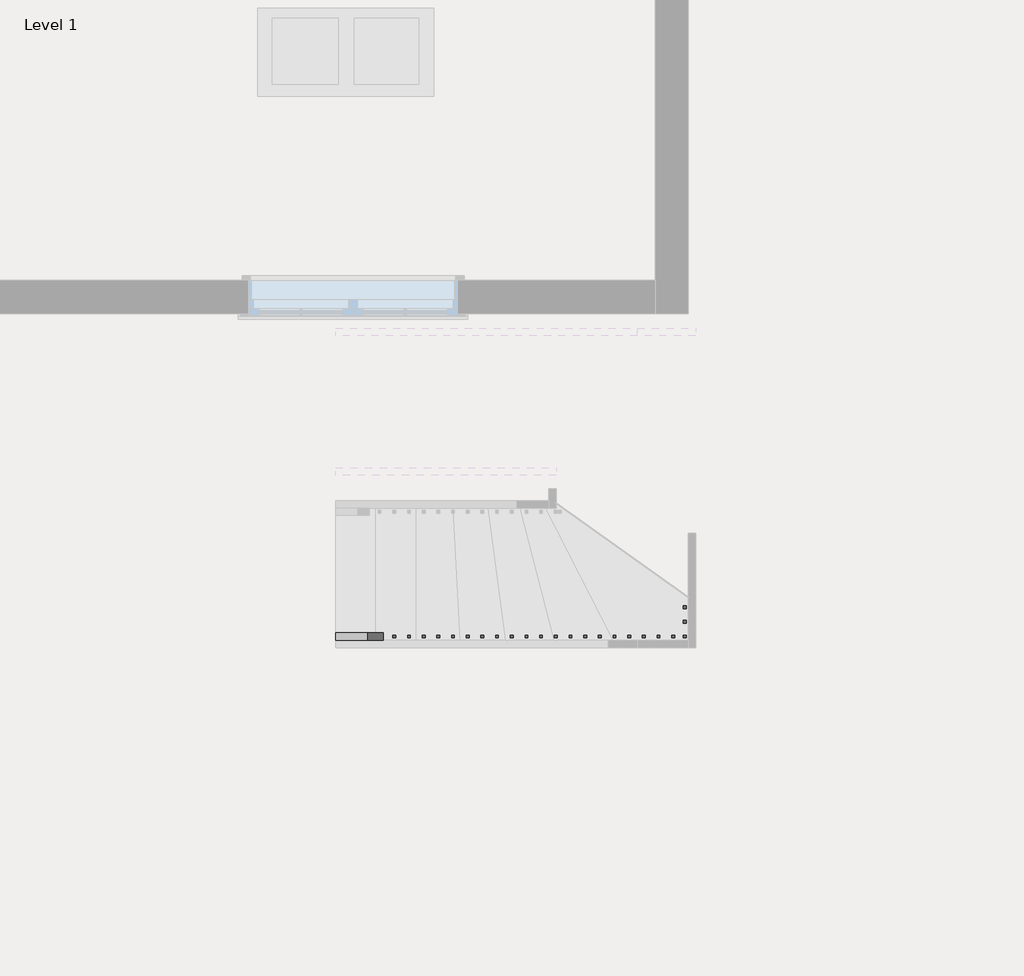
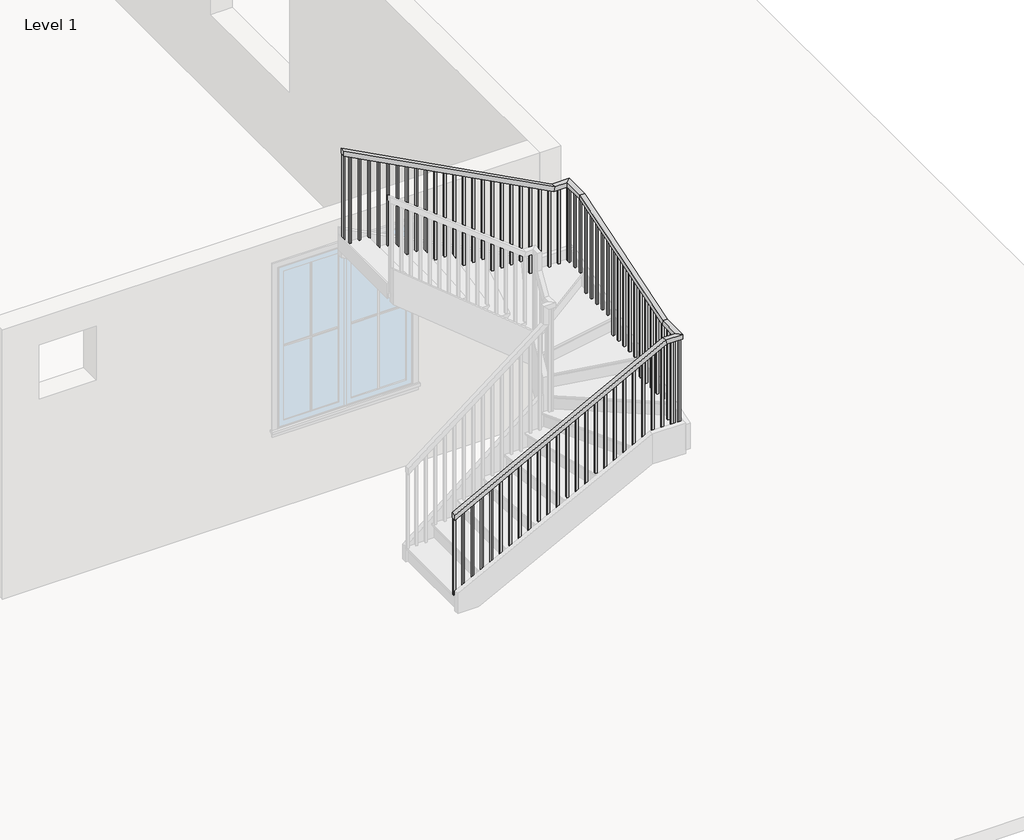
# One storey, part 2 of 3: 1 railing.
"""IFC4 building model written with IfcOpenShell, lengths in millimetres."""

from ifc_helpers import new_model, si_unit, frame, origin, place, context, project, spatial, polyline, outline, extrude, faceted_brep, element, save

model = new_model("IFC4")

# Units and contexts
model_context = context("Model", 3, world=origin())
ifc_project = project(units=[si_unit("LENGTHUNIT", "METRE", prefix="MILLI")], contexts=[model_context])

# Site, building, storey
site = spatial("IfcSite", under=ifc_project)
building = spatial("IfcBuilding", under=site)
storey = spatial("IfcBuildingStorey", under=building, Name="Level 1", Elevation=0.0)

# Railing
placement = place(None, origin())
element("IfcRailing", 1, ObjectType="Handrail - Rectangular", at=placement, inside=storey, context=model_context, shape_type="SolidModel", body=[
    faceted_brep([(531.7538115, -7514.4090409, 1083.7333333), (531.7538115, -7514.4090409, 1026.2742652), (531.7538115, -7565.2090409, 1026.2742652), (531.7538115, -7565.2090409, 1083.7333333), (2789.4788736, -7514.4090409, 2277.0239201), (2802.0779381, -7514.4090409, 2226.2239201), (2802.0779381, -7565.2090409, 2226.2239201), (2789.4788736, -7565.2090409, 2277.0239201), (2923.0855034, -7269.9465826, 2226.2239201), (2923.0855034, -7277.8971587, 2277.0239201), (2923.0855034, -5744.320923, 2769.1094132), (2923.0855034, -5736.3703469, 2718.3094132), (2973.8855034, -7269.9465826, 2226.2239201), (2973.8855034, -5736.3703469, 2718.3094132), (2973.8855034, -7277.8971587, 2277.0239201), (2973.8855034, -5744.320923, 2769.1094132), (531.7538115, -5507.8090409, 3962.4), (531.7538115, -5457.0090409, 3962.4), (531.7538115, -5457.0090409, 3904.9409318), (531.7538115, -5507.8090409, 3904.9409318), (2776.879809, -5507.8090409, 2718.3094132), (2789.4788736, -5507.8090409, 2769.1094132), (2776.879809, -5457.0090409, 2718.3094132), (2789.4788736, -5457.0090409, 2769.1094132), (2923.0855034, -7514.4090409, 2277.0239201), (2923.0855034, -7514.4090409, 2226.2239201), (2973.8855034, -7565.2090409, 2226.2239201), (2973.8855034, -7565.2090409, 2277.0239201), (2923.0855034, -5507.8090409, 2769.1094132), (2923.0855034, -5507.8090409, 2718.3094132), (2973.8855034, -5457.0090409, 2718.3094132), (2973.8855034, -5457.0090409, 2769.1094132)], [[[0, 1, 2, 3]], [[1, 0, 4, 5]], [[2, 1, 5, 6]], [[3, 2, 6, 7]], [[0, 3, 7, 4]], [[8, 9, 10, 11]], [[12, 8, 11, 13]], [[14, 12, 13, 15]], [[9, 14, 15, 10]], [[16, 17, 18, 19]], [[20, 21, 16, 19]], [[22, 20, 19, 18]], [[23, 22, 18, 17]], [[21, 23, 17, 16]], [[5, 4, 24, 25]], [[6, 5, 25, 26]], [[7, 6, 26, 27]], [[4, 7, 27, 24]], [[25, 24, 9, 8]], [[26, 25, 8, 12]], [[27, 26, 12, 14]], [[24, 27, 14, 9]], [[11, 10, 28, 29]], [[13, 11, 29, 30]], [[15, 13, 30, 31]], [[10, 15, 31, 28]], [[29, 28, 21, 20]], [[30, 29, 20, 22]], [[31, 30, 22, 23]], [[28, 31, 23, 21]]]),
    extrude(outline(polyline([(3857.6597858, 621.2105034), (3867.7284102, 602.1605034), (2878.6666667, 602.1605034), (2878.6666667, 621.2105034), (3857.6597858, 621.2105034)])), frame((0.0, -5491.9340409, 0.0), z_axis=(0.0, 1.0, 0.0), x_axis=(0.0, 0.0, 1.0)), (0.0, 0.0, 1.0), 19.05),
    extrude(outline(polyline([(3803.9604556, 722.8105034), (3814.02908, 703.7605034), (2878.6666667, 703.7605034), (2878.6666667, 722.8105034), (3803.9604556, 722.8105034)])), frame((0.0, -5491.9340409, 0.0), z_axis=(0.0, 1.0, 0.0), x_axis=(0.0, 0.0, 1.0)), (0.0, 0.0, 1.0), 19.05),
    extrude(outline(polyline([(3750.2611254, 824.4105034), (3760.3297498, 805.3605034), (2709.3333333, 805.3605034), (2709.3333333, 824.4105034), (3750.2611254, 824.4105034)])), frame((0.0, -5491.9340409, 0.0), z_axis=(0.0, 1.0, 0.0), x_axis=(0.0, 0.0, 1.0)), (0.0, 0.0, 1.0), 19.05),
    extrude(outline(polyline([(3696.5617952, 926.0105034), (3706.6304196, 906.9605034), (2709.3333333, 906.9605034), (2709.3333333, 926.0105034), (3696.5617952, 926.0105034)])), frame((0.0, -5491.9340409, 0.0), z_axis=(0.0, 1.0, 0.0), x_axis=(0.0, 0.0, 1.0)), (0.0, 0.0, 1.0), 19.05),
    extrude(outline(polyline([(3642.862465, 1027.6105034), (3652.9310894, 1008.5605034), (2709.3333333, 1008.5605034), (2709.3333333, 1027.6105034), (3642.862465, 1027.6105034)])), frame((0.0, -5491.9340409, 0.0), z_axis=(0.0, 1.0, 0.0), x_axis=(0.0, 0.0, 1.0)), (0.0, 0.0, 1.0), 19.05),
    extrude(outline(polyline([(3589.1631348, 1129.2105034), (3599.2317592, 1110.1605034), (2540.0, 1110.1605034), (2540.0, 1129.2105034), (3589.1631348, 1129.2105034)])), frame((0.0, -5491.9340409, 0.0), z_axis=(0.0, 1.0, 0.0), x_axis=(0.0, 0.0, 1.0)), (0.0, 0.0, 1.0), 19.05),
    extrude(outline(polyline([(3535.4638046, 1230.8105034), (3545.532429, 1211.7605034), (2540.0, 1211.7605034), (2540.0, 1230.8105034), (3535.4638046, 1230.8105034)])), frame((0.0, -5491.9340409, 0.0), z_axis=(0.0, 1.0, 0.0), x_axis=(0.0, 0.0, 1.0)), (0.0, 0.0, 1.0), 19.05),
    extrude(outline(polyline([(3481.7644744, 1332.4105034), (3491.8330988, 1313.3605034), (2540.0, 1313.3605034), (2540.0, 1332.4105034), (3481.7644744, 1332.4105034)])), frame((0.0, -5491.9340409, 0.0), z_axis=(0.0, 1.0, 0.0), x_axis=(0.0, 0.0, 1.0)), (0.0, 0.0, 1.0), 19.05),
    extrude(outline(polyline([(3428.0651442, 1434.0105034), (3438.1337686, 1414.9605034), (2370.6666667, 1414.9605034), (2370.6666667, 1434.0105034), (3428.0651442, 1434.0105034)])), frame((0.0, -5491.9340409, 0.0), z_axis=(0.0, 1.0, 0.0), x_axis=(0.0, 0.0, 1.0)), (0.0, 0.0, 1.0), 19.05),
    extrude(outline(polyline([(3374.365814, 1535.6105034), (3384.4344384, 1516.5605034), (2370.6666667, 1516.5605034), (2370.6666667, 1535.6105034), (3374.365814, 1535.6105034)])), frame((0.0, -5491.9340409, 0.0), z_axis=(0.0, 1.0, 0.0), x_axis=(0.0, 0.0, 1.0)), (0.0, 0.0, 1.0), 19.05),
    extrude(outline(polyline([(3320.6664838, 1637.2105034), (3330.7351082, 1618.1605034), (2370.6666667, 1618.1605034), (2370.6666667, 1637.2105034), (3320.6664838, 1637.2105034)])), frame((0.0, -5491.9340409, 0.0), z_axis=(0.0, 1.0, 0.0), x_axis=(0.0, 0.0, 1.0)), (0.0, 0.0, 1.0), 19.05),
    extrude(outline(polyline([(3266.9671536, 1738.8105034), (3277.035778, 1719.7605034), (2201.3333333, 1719.7605034), (2201.3333333, 1738.8105034), (3266.9671536, 1738.8105034)])), frame((0.0, -5491.9340409, 0.0), z_axis=(0.0, 1.0, 0.0), x_axis=(0.0, 0.0, 1.0)), (0.0, 0.0, 1.0), 19.05),
    extrude(outline(polyline([(3213.2678234, 1840.4105034), (3223.3364478, 1821.3605034), (2201.3333333, 1821.3605034), (2201.3333333, 1840.4105034), (3213.2678234, 1840.4105034)])), frame((0.0, -5491.9340409, 0.0), z_axis=(0.0, 1.0, 0.0), x_axis=(0.0, 0.0, 1.0)), (0.0, 0.0, 1.0), 19.05),
    extrude(outline(polyline([(3159.5684932, 1942.0105034), (3169.6371176, 1922.9605034), (2201.3333333, 1922.9605034), (2201.3333333, 1942.0105034), (3159.5684932, 1942.0105034)])), frame((0.0, -5491.9340409, 0.0), z_axis=(0.0, 1.0, 0.0), x_axis=(0.0, 0.0, 1.0)), (0.0, 0.0, 1.0), 19.05),
    extrude(outline(polyline([(3105.869163, 2043.6105034), (3115.9377874, 2024.5605034), (2201.3333333, 2024.5605034), (2201.3333333, 2043.6105034), (3105.869163, 2043.6105034)])), frame((0.0, -5491.9340409, 0.0), z_axis=(0.0, 1.0, 0.0), x_axis=(0.0, 0.0, 1.0)), (0.0, 0.0, 1.0), 19.05),
    extrude(outline(polyline([(3052.1698328, 2145.2105034), (3062.2384572, 2126.1605034), (2032.0, 2126.1605034), (2032.0, 2145.2105034), (3052.1698328, 2145.2105034)])), frame((0.0, -5491.9340409, 0.0), z_axis=(0.0, 1.0, 0.0), x_axis=(0.0, 0.0, 1.0)), (0.0, 0.0, 1.0), 19.05),
    extrude(outline(polyline([(2998.4705026, 2246.8105034), (3008.539127, 2227.7605034), (2032.0, 2227.7605034), (2032.0, 2246.8105034), (2998.4705026, 2246.8105034)])), frame((0.0, -5491.9340409, 0.0), z_axis=(0.0, 1.0, 0.0), x_axis=(0.0, 0.0, 1.0)), (0.0, 0.0, 1.0), 19.05),
    extrude(outline(polyline([(2944.7711724, 2348.4105034), (2954.8397968, 2329.3605034), (2032.0, 2329.3605034), (2032.0, 2348.4105034), (2944.7711724, 2348.4105034)])), frame((0.0, -5491.9340409, 0.0), z_axis=(0.0, 1.0, 0.0), x_axis=(0.0, 0.0, 1.0)), (0.0, 0.0, 1.0), 19.05),
    extrude(outline(polyline([(2891.0718422, 2450.0105034), (2901.1404666, 2430.9605034), (2032.0, 2430.9605034), (2032.0, 2450.0105034), (2891.0718422, 2450.0105034)])), frame((0.0, -5491.9340409, 0.0), z_axis=(0.0, 1.0, 0.0), x_axis=(0.0, 0.0, 1.0)), (0.0, 0.0, 1.0), 19.05),
    extrude(outline(polyline([(2837.372512, 2551.6105034), (2847.4411364, 2532.5605034), (1862.6666667, 2532.5605034), (1862.6666667, 2551.6105034), (2837.372512, 2551.6105034)])), frame((0.0, -5491.9340409, 0.0), z_axis=(0.0, 1.0, 0.0), x_axis=(0.0, 0.0, 1.0)), (0.0, 0.0, 1.0), 19.05),
    extrude(outline(polyline([(2783.6731818, 2653.2105034), (2793.7418062, 2634.1605034), (1862.6666667, 2634.1605034), (1862.6666667, 2653.2105034), (2783.6731818, 2653.2105034)])), frame((0.0, -5491.9340409, 0.0), z_axis=(0.0, 1.0, 0.0), x_axis=(0.0, 0.0, 1.0)), (0.0, 0.0, 1.0), 19.05),
    extrude(outline(polyline([(2729.9738516, 2754.8105034), (2740.042476, 2735.7605034), (1862.6666667, 2735.7605034), (1862.6666667, 2754.8105034), (2729.9738516, 2754.8105034)])), frame((0.0, -5491.9340409, 0.0), z_axis=(0.0, 1.0, 0.0), x_axis=(0.0, 0.0, 1.0)), (0.0, 0.0, 1.0), 19.05),
    extrude(outline(polyline([(2856.4105034, -5472.8840409), (2856.4105034, -5491.9340409), (2837.3605034, -5491.9340409), (2837.3605034, -5472.8840409), (2856.4105034, -5472.8840409)])), frame((0.0, 0.0, 1862.6666667), z_axis=(0.0, 0.0, 1.0), x_axis=(1.0, 0.0, 0.0)), (0.0, 0.0, 1.0), 855.6427466),
    extrude(outline(polyline([(2958.0105034, -5517.3340409), (2938.9605034, -5517.3340409), (2938.9605034, -5498.2840409), (2958.0105034, -5498.2840409), (2958.0105034, -5517.3340409)])), frame((0.0, 0.0, 1862.6666667), z_axis=(0.0, 0.0, 1.0), x_axis=(1.0, 0.0, 0.0)), (0.0, 0.0, 1.0), 855.6427466),
    extrude(outline(polyline([(2958.0105034, -5618.9340409), (2938.9605034, -5618.9340409), (2938.9605034, -5599.8840409), (2958.0105034, -5599.8840409), (2958.0105034, -5618.9340409)])), frame((0.0, 0.0, 1862.6666667), z_axis=(0.0, 0.0, 1.0), x_axis=(1.0, 0.0, 0.0)), (0.0, 0.0, 1.0), 855.6427466),
    extrude(outline(polyline([(2958.0105034, -5720.5340409), (2938.9605034, -5720.5340409), (2938.9605034, -5701.4840409), (2958.0105034, -5701.4840409), (2958.0105034, -5720.5340409)])), frame((0.0, 0.0, 1862.6666667), z_axis=(0.0, 0.0, 1.0), x_axis=(1.0, 0.0, 0.0)), (0.0, 0.0, 1.0), 855.6427466),
    extrude(outline(polyline([(-5822.1340409, 2690.7900316), (-5803.0840409, 2696.9026907), (-5803.0840409, 1693.3333333), (-5822.1340409, 1693.3333333), (-5822.1340409, 2690.7900316)])), frame((2938.9605034, 0.0, 0.0), z_axis=(1.0, 0.0, 0.0), x_axis=(0.0, 1.0, 0.0)), (0.0, 0.0, 1.0), 19.05),
    extrude(outline(polyline([(-5923.7340409, 2658.1891834), (-5904.6840409, 2664.3018425), (-5904.6840409, 1693.3333333), (-5923.7340409, 1693.3333333), (-5923.7340409, 2658.1891834)])), frame((2938.9605034, 0.0, 0.0), z_axis=(1.0, 0.0, 0.0), x_axis=(0.0, 1.0, 0.0)), (0.0, 0.0, 1.0), 19.05),
    extrude(outline(polyline([(-6025.3340409, 2625.5883352), (-6006.2840409, 2631.7009942), (-6006.2840409, 1693.3333333), (-6025.3340409, 1693.3333333), (-6025.3340409, 2625.5883352)])), frame((2938.9605034, 0.0, 0.0), z_axis=(1.0, 0.0, 0.0), x_axis=(0.0, 1.0, 0.0)), (0.0, 0.0, 1.0), 19.05),
    extrude(outline(polyline([(-6126.9340409, 2592.987487), (-6107.8840409, 2599.100146), (-6107.8840409, 1693.3333333), (-6126.9340409, 1693.3333333), (-6126.9340409, 2592.987487)])), frame((2938.9605034, 0.0, 0.0), z_axis=(1.0, 0.0, 0.0), x_axis=(0.0, 1.0, 0.0)), (0.0, 0.0, 1.0), 19.05),
    extrude(outline(polyline([(-6228.5340409, 2560.3866387), (-6209.4840409, 2566.4992978), (-6209.4840409, 1693.3333333), (-6228.5340409, 1693.3333333), (-6228.5340409, 2560.3866387)])), frame((2938.9605034, 0.0, 0.0), z_axis=(1.0, 0.0, 0.0), x_axis=(0.0, 1.0, 0.0)), (0.0, 0.0, 1.0), 19.05),
    extrude(outline(polyline([(-6330.1340409, 2527.7857905), (-6311.0840409, 2533.8984495), (-6311.0840409, 1524.0), (-6330.1340409, 1524.0), (-6330.1340409, 2527.7857905)])), frame((2938.9605034, 0.0, 0.0), z_axis=(1.0, 0.0, 0.0), x_axis=(0.0, 1.0, 0.0)), (0.0, 0.0, 1.0), 19.05),
    extrude(outline(polyline([(-6431.7340409, 2495.1849423), (-6412.6840409, 2501.2976013), (-6412.6840409, 1524.0), (-6431.7340409, 1524.0), (-6431.7340409, 2495.1849423)])), frame((2938.9605034, 0.0, 0.0), z_axis=(1.0, 0.0, 0.0), x_axis=(0.0, 1.0, 0.0)), (0.0, 0.0, 1.0), 19.05),
    extrude(outline(polyline([(-6533.3340409, 2462.5840941), (-6514.2840409, 2468.6967531), (-6514.2840409, 1524.0), (-6533.3340409, 1524.0), (-6533.3340409, 2462.5840941)])), frame((2938.9605034, 0.0, 0.0), z_axis=(1.0, 0.0, 0.0), x_axis=(0.0, 1.0, 0.0)), (0.0, 0.0, 1.0), 19.05),
    extrude(outline(polyline([(-6634.9340409, 2429.9832458), (-6615.8840409, 2436.0959049), (-6615.8840409, 1524.0), (-6634.9340409, 1524.0), (-6634.9340409, 2429.9832458)])), frame((2938.9605034, 0.0, 0.0), z_axis=(1.0, 0.0, 0.0), x_axis=(0.0, 1.0, 0.0)), (0.0, 0.0, 1.0), 19.05),
    extrude(outline(polyline([(-6736.5340409, 2397.3823976), (-6717.4840409, 2403.4950566), (-6717.4840409, 1524.0), (-6736.5340409, 1524.0), (-6736.5340409, 2397.3823976)])), frame((2938.9605034, 0.0, 0.0), z_axis=(1.0, 0.0, 0.0), x_axis=(0.0, 1.0, 0.0)), (0.0, 0.0, 1.0), 19.05),
    extrude(outline(polyline([(-6838.1340409, 2364.7815494), (-6819.0840409, 2370.8942084), (-6819.0840409, 1354.6666667), (-6838.1340409, 1354.6666667), (-6838.1340409, 2364.7815494)])), frame((2938.9605034, 0.0, 0.0), z_axis=(1.0, 0.0, 0.0), x_axis=(0.0, 1.0, 0.0)), (0.0, 0.0, 1.0), 19.05),
    extrude(outline(polyline([(-6939.7340409, 2332.1807011), (-6920.6840409, 2338.2933602), (-6920.6840409, 1354.6666667), (-6939.7340409, 1354.6666667), (-6939.7340409, 2332.1807011)])), frame((2938.9605034, 0.0, 0.0), z_axis=(1.0, 0.0, 0.0), x_axis=(0.0, 1.0, 0.0)), (0.0, 0.0, 1.0), 19.05),
    extrude(outline(polyline([(-7041.3340409, 2299.5798529), (-7022.2840409, 2305.692512), (-7022.2840409, 1354.6666667), (-7041.3340409, 1354.6666667), (-7041.3340409, 2299.5798529)])), frame((2938.9605034, 0.0, 0.0), z_axis=(1.0, 0.0, 0.0), x_axis=(0.0, 1.0, 0.0)), (0.0, 0.0, 1.0), 19.05),
    extrude(outline(polyline([(-7142.9340409, 2266.9790047), (-7123.8840409, 2273.0916637), (-7123.8840409, 1354.6666667), (-7142.9340409, 1354.6666667), (-7142.9340409, 2266.9790047)])), frame((2938.9605034, 0.0, 0.0), z_axis=(1.0, 0.0, 0.0), x_axis=(0.0, 1.0, 0.0)), (0.0, 0.0, 1.0), 19.05),
    extrude(outline(polyline([(-7244.5340409, 2234.3781565), (-7225.4840409, 2240.4908155), (-7225.4840409, 1354.6666667), (-7244.5340409, 1354.6666667), (-7244.5340409, 2234.3781565)])), frame((2938.9605034, 0.0, 0.0), z_axis=(1.0, 0.0, 0.0), x_axis=(0.0, 1.0, 0.0)), (0.0, 0.0, 1.0), 19.05),
    extrude(outline(polyline([(2958.0105034, -7346.1340409), (2938.9605034, -7346.1340409), (2938.9605034, -7327.0840409), (2958.0105034, -7327.0840409), (2958.0105034, -7346.1340409)])), frame((0.0, 0.0, 1185.3333333), z_axis=(0.0, 0.0, 1.0), x_axis=(1.0, 0.0, 0.0)), (0.0, 0.0, 1.0), 1040.8905868),
    extrude(outline(polyline([(2958.0105034, -7447.7340409), (2938.9605034, -7447.7340409), (2938.9605034, -7428.6840409), (2958.0105034, -7428.6840409), (2958.0105034, -7447.7340409)])), frame((0.0, 0.0, 1185.3333333), z_axis=(0.0, 0.0, 1.0), x_axis=(1.0, 0.0, 0.0)), (0.0, 0.0, 1.0), 1040.8905868),
    extrude(outline(polyline([(2859.0288115, -7549.3340409), (2859.0288115, -7530.2840409), (2878.0788115, -7530.2840409), (2878.0788115, -7549.3340409), (2859.0288115, -7549.3340409)])), frame((0.0, 0.0, 1185.3333333), z_axis=(0.0, 0.0, 1.0), x_axis=(1.0, 0.0, 0.0)), (0.0, 0.0, 1.0), 1040.8905868),
    extrude(outline(polyline([(2212.6938418, 2776.4788115), (2202.6252174, 2757.4288115), (1185.3333333, 2757.4288115), (1185.3333333, 2776.4788115), (2212.6938418, 2776.4788115)])), frame((0.0, -7549.3340409, 0.0), z_axis=(0.0, 1.0, 0.0), x_axis=(0.0, 0.0, 1.0)), (0.0, 0.0, 1.0), 19.05),
    extrude(outline(polyline([(2158.9945116, 2674.8788115), (2148.9258872, 2655.8288115), (1185.3333333, 2655.8288115), (1185.3333333, 2674.8788115), (2158.9945116, 2674.8788115)])), frame((0.0, -7549.3340409, 0.0), z_axis=(0.0, 1.0, 0.0), x_axis=(0.0, 0.0, 1.0)), (0.0, 0.0, 1.0), 19.05),
    extrude(outline(polyline([(2105.2951814, 2573.2788115), (2095.226557, 2554.2288115), (1185.3333333, 2554.2288115), (1185.3333333, 2573.2788115), (2105.2951814, 2573.2788115)])), frame((0.0, -7549.3340409, 0.0), z_axis=(0.0, 1.0, 0.0), x_axis=(0.0, 0.0, 1.0)), (0.0, 0.0, 1.0), 19.05),
    extrude(outline(polyline([(2051.5958512, 2471.6788115), (2041.5272268, 2452.6288115), (1185.3333333, 2452.6288115), (1185.3333333, 2471.6788115), (2051.5958512, 2471.6788115)])), frame((0.0, -7549.3340409, 0.0), z_axis=(0.0, 1.0, 0.0), x_axis=(0.0, 0.0, 1.0)), (0.0, 0.0, 1.0), 19.05),
    extrude(outline(polyline([(1997.896521, 2370.0788115), (1987.8278966, 2351.0288115), (1016.0, 2351.0288115), (1016.0, 2370.0788115), (1997.896521, 2370.0788115)])), frame((0.0, -7549.3340409, 0.0), z_axis=(0.0, 1.0, 0.0), x_axis=(0.0, 0.0, 1.0)), (0.0, 0.0, 1.0), 19.05),
    extrude(outline(polyline([(1944.1971908, 2268.4788115), (1934.1285664, 2249.4288115), (1016.0, 2249.4288115), (1016.0, 2268.4788115), (1944.1971908, 2268.4788115)])), frame((0.0, -7549.3340409, 0.0), z_axis=(0.0, 1.0, 0.0), x_axis=(0.0, 0.0, 1.0)), (0.0, 0.0, 1.0), 19.05),
    extrude(outline(polyline([(1890.4978606, 2166.8788115), (1880.4292362, 2147.8288115), (1016.0, 2147.8288115), (1016.0, 2166.8788115), (1890.4978606, 2166.8788115)])), frame((0.0, -7549.3340409, 0.0), z_axis=(0.0, 1.0, 0.0), x_axis=(0.0, 0.0, 1.0)), (0.0, 0.0, 1.0), 19.05),
    extrude(outline(polyline([(1836.7985304, 2065.2788115), (1826.729906, 2046.2288115), (1016.0, 2046.2288115), (1016.0, 2065.2788115), (1836.7985304, 2065.2788115)])), frame((0.0, -7549.3340409, 0.0), z_axis=(0.0, 1.0, 0.0), x_axis=(0.0, 0.0, 1.0)), (0.0, 0.0, 1.0), 19.05),
    extrude(outline(polyline([(1783.0992002, 1963.6788115), (1773.0305758, 1944.6288115), (846.6666667, 1944.6288115), (846.6666667, 1963.6788115), (1783.0992002, 1963.6788115)])), frame((0.0, -7549.3340409, 0.0), z_axis=(0.0, 1.0, 0.0), x_axis=(0.0, 0.0, 1.0)), (0.0, 0.0, 1.0), 19.05),
    extrude(outline(polyline([(1729.39987, 1862.0788115), (1719.3312456, 1843.0288115), (846.6666667, 1843.0288115), (846.6666667, 1862.0788115), (1729.39987, 1862.0788115)])), frame((0.0, -7549.3340409, 0.0), z_axis=(0.0, 1.0, 0.0), x_axis=(0.0, 0.0, 1.0)), (0.0, 0.0, 1.0), 19.05),
    extrude(outline(polyline([(1675.7005398, 1760.4788115), (1665.6319154, 1741.4288115), (846.6666667, 1741.4288115), (846.6666667, 1760.4788115), (1675.7005398, 1760.4788115)])), frame((0.0, -7549.3340409, 0.0), z_axis=(0.0, 1.0, 0.0), x_axis=(0.0, 0.0, 1.0)), (0.0, 0.0, 1.0), 19.05),
    extrude(outline(polyline([(1622.0012096, 1658.8788115), (1611.9325852, 1639.8288115), (677.3333333, 1639.8288115), (677.3333333, 1658.8788115), (1622.0012096, 1658.8788115)])), frame((0.0, -7549.3340409, 0.0), z_axis=(0.0, 1.0, 0.0), x_axis=(0.0, 0.0, 1.0)), (0.0, 0.0, 1.0), 19.05),
    extrude(outline(polyline([(1568.3018794, 1557.2788115), (1558.233255, 1538.2288115), (677.3333333, 1538.2288115), (677.3333333, 1557.2788115), (1568.3018794, 1557.2788115)])), frame((0.0, -7549.3340409, 0.0), z_axis=(0.0, 1.0, 0.0), x_axis=(0.0, 0.0, 1.0)), (0.0, 0.0, 1.0), 19.05),
    extrude(outline(polyline([(1514.6025492, 1455.6788115), (1504.5339248, 1436.6288115), (677.3333333, 1436.6288115), (677.3333333, 1455.6788115), (1514.6025492, 1455.6788115)])), frame((0.0, -7549.3340409, 0.0), z_axis=(0.0, 1.0, 0.0), x_axis=(0.0, 0.0, 1.0)), (0.0, 0.0, 1.0), 19.05),
    extrude(outline(polyline([(1460.903219, 1354.0788115), (1450.8345946, 1335.0288115), (508.0, 1335.0288115), (508.0, 1354.0788115), (1460.903219, 1354.0788115)])), frame((0.0, -7549.3340409, 0.0), z_axis=(0.0, 1.0, 0.0), x_axis=(0.0, 0.0, 1.0)), (0.0, 0.0, 1.0), 19.05),
    extrude(outline(polyline([(1407.2038888, 1252.4788115), (1397.1352644, 1233.4288115), (508.0, 1233.4288115), (508.0, 1252.4788115), (1407.2038888, 1252.4788115)])), frame((0.0, -7549.3340409, 0.0), z_axis=(0.0, 1.0, 0.0), x_axis=(0.0, 0.0, 1.0)), (0.0, 0.0, 1.0), 19.05),
    extrude(outline(polyline([(1353.5045586, 1150.8788115), (1343.4359342, 1131.8288115), (508.0, 1131.8288115), (508.0, 1150.8788115), (1353.5045586, 1150.8788115)])), frame((0.0, -7549.3340409, 0.0), z_axis=(0.0, 1.0, 0.0), x_axis=(0.0, 0.0, 1.0)), (0.0, 0.0, 1.0), 19.05),
    extrude(outline(polyline([(1299.8052284, 1049.2788115), (1289.736604, 1030.2288115), (338.6666667, 1030.2288115), (338.6666667, 1049.2788115), (1299.8052284, 1049.2788115)])), frame((0.0, -7549.3340409, 0.0), z_axis=(0.0, 1.0, 0.0), x_axis=(0.0, 0.0, 1.0)), (0.0, 0.0, 1.0), 19.05),
    extrude(outline(polyline([(1246.1058982, 947.6788115), (1236.0372738, 928.6288115), (338.6666667, 928.6288115), (338.6666667, 947.6788115), (1246.1058982, 947.6788115)])), frame((0.0, -7549.3340409, 0.0), z_axis=(0.0, 1.0, 0.0), x_axis=(0.0, 0.0, 1.0)), (0.0, 0.0, 1.0), 19.05),
    extrude(outline(polyline([(1192.406568, 846.0788115), (1182.3379436, 827.0288115), (338.6666667, 827.0288115), (338.6666667, 846.0788115), (1192.406568, 846.0788115)])), frame((0.0, -7549.3340409, 0.0), z_axis=(0.0, 1.0, 0.0), x_axis=(0.0, 0.0, 1.0)), (0.0, 0.0, 1.0), 19.05),
    extrude(outline(polyline([(1138.7072378, 744.4788115), (1128.6386134, 725.4288115), (169.3333333, 725.4288115), (169.3333333, 744.4788115), (1138.7072378, 744.4788115)])), frame((0.0, -7549.3340409, 0.0), z_axis=(0.0, 1.0, 0.0), x_axis=(0.0, 0.0, 1.0)), (0.0, 0.0, 1.0), 19.05),
    extrude(outline(polyline([(1085.0079076, 642.8788115), (1074.9392831, 623.8288115), (169.3333333, 623.8288115), (169.3333333, 642.8788115), (1085.0079076, 642.8788115)])), frame((0.0, -7549.3340409, 0.0), z_axis=(0.0, 1.0, 0.0), x_axis=(0.0, 0.0, 1.0)), (0.0, 0.0, 1.0), 19.05),
    extrude(outline(polyline([(2958.0105034, -5491.9340409), (2938.9605034, -5491.9340409), (2938.9605034, -5472.8840409), (2958.0105034, -5472.8840409), (2958.0105034, -5491.9340409)])), frame((0.0, 0.0, 1862.6666667), z_axis=(0.0, 0.0, 1.0), x_axis=(1.0, 0.0, 0.0)), (0.0, 0.0, 1.0), 855.6427466),
    extrude(outline(polyline([(2938.9605034, -7549.3340409), (2938.9605034, -7530.2840409), (2958.0105034, -7530.2840409), (2958.0105034, -7549.3340409), (2938.9605034, -7549.3340409)])), frame((0.0, 0.0, 1185.3333333), z_axis=(0.0, 0.0, 1.0), x_axis=(1.0, 0.0, 0.0)), (0.0, 0.0, 1.0), 1040.8905868),
    extrude(outline(polyline([(3894.8723074, 550.8038115), (3904.9409318, 531.7538115), (2878.6666667, 531.7538115), (2878.6666667, 550.8038115), (3894.8723074, 550.8038115)])), frame((0.0, -5491.9340409, 0.0), z_axis=(0.0, 1.0, 0.0), x_axis=(0.0, 0.0, 1.0)), (0.0, 0.0, 1.0), 19.05),
    extrude(outline(polyline([(1036.3428896, 550.8038115), (1026.2742652, 531.7538115), (169.3333333, 531.7538115), (169.3333333, 550.8038115), (1036.3428896, 550.8038115)])), frame((0.0, -7549.3340409, 0.0), z_axis=(0.0, 1.0, 0.0), x_axis=(0.0, 0.0, 1.0)), (0.0, 0.0, 1.0), 19.05),
])

save(model, "model.ifc")

# Revit data of these elements
# Type "Handrail - Rectangular"
#   Assembly Code = "C2010400"
#   built-in parameter 1008612 = 0.0416667 (stored number, unit not read)
#   built-in parameter 1008611 = 0.0416667 (stored number, unit not read)
#   built-in parameter 1008609 = 0.333333 (stored number, unit not read)
#   built-in parameter 1008604 = 0.166667 (stored number, unit not read)
#   built-in parameter 1008603 = 0.166667 (stored number, unit not read)
#   Railing Height = 3' - 0"
#   built-in parameter 1008630 = 2
#   built-in parameter 1008610 = 2
#   built-in parameter 1008618 = Baluster - Square : 3/4"
# Element 1 (IfcRailing, "Handrail - Rectangular")
#   Phase Created = New Construction
